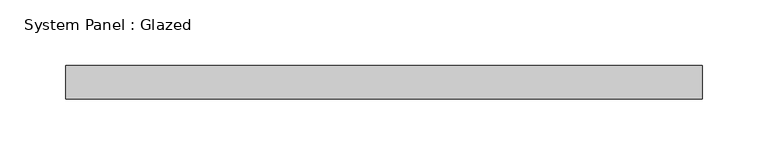
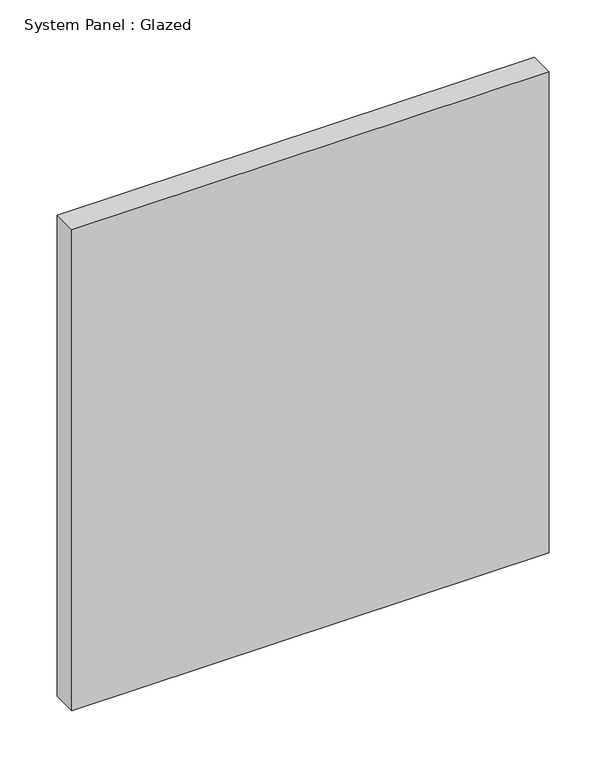
"""IFC4 building model written with IfcOpenShell, lengths in millimetres: plate geometry, System Panel : Glazed."""

from ifc_helpers import new_model, si_unit, origin, origin_with_axes, place, context, project, spatial, polyline, outline, extrude, source, transform, mapped, element, save


def system_panel_glazed_c43f0a09(model_context):
    return source(origin(), model_context, "Body", "SweptSolid", [
        extrude(outline(polyline([(241.3, 19.05), (-241.3, 19.05), (-241.3, 44.45), (241.3, 44.45), (241.3, 19.05)])), origin_with_axes(), (0.0, 0.0, 1.0), 514.35),
    ])


if __name__ == "__main__":
    model = new_model("IFC4")
    model_context = context("Model", 3, world=origin())
    ifc_project = project(units=[si_unit("LENGTHUNIT", "METRE", prefix="MILLI")], contexts=[model_context])
    site = spatial("IfcSite", under=ifc_project)
    building = spatial("IfcBuilding", under=site)
    placement = place(None, origin())
    system_panel_glazed_shape = system_panel_glazed_c43f0a09(model_context)
    element("IfcPlate", 1, ObjectType="System Panel : Glazed", at=placement, inside=building, context=model_context, shape_type="MappedRepresentation", body=[
        mapped(system_panel_glazed_shape, transform((0.0, 0.0, 0.0), x_axis=(1.0, 0.0, 0.0), y_axis=(0.0, 1.0, 0.0), z_axis=(0.0, 0.0, 1.0))),
    ])
    save(model, "model.ifc")

# Revit data of these elements
# Type "System Panel : Glazed"
#   Construction Type Id = "GSP4R"
#   Analytic Construction = "1/8 in Pilkington single glazing"
#   Visual Light Transmittance = 0.9
#   Solar Heat Gain Coefficient = 0.86
#   Heat Transfer Coefficient (U) = 1.18115 BTU/(h·ft²·°F)
#   Define Thermal Properties by = 1
# Element 1 (IfcPlate, "System Panel : Glazed")
#   Materials on its faces: "Glass"
# Materials
#   "Glass": class "Glass", colour RGB 0 128 192, transparency 0.75, Description = "Soda Lime Glass", Cost = 0
